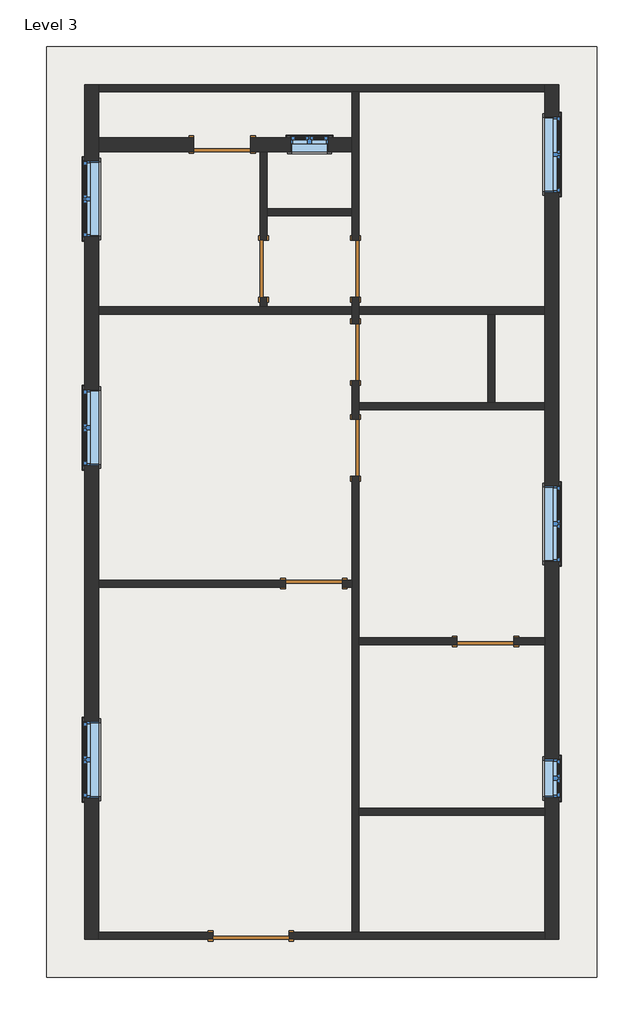
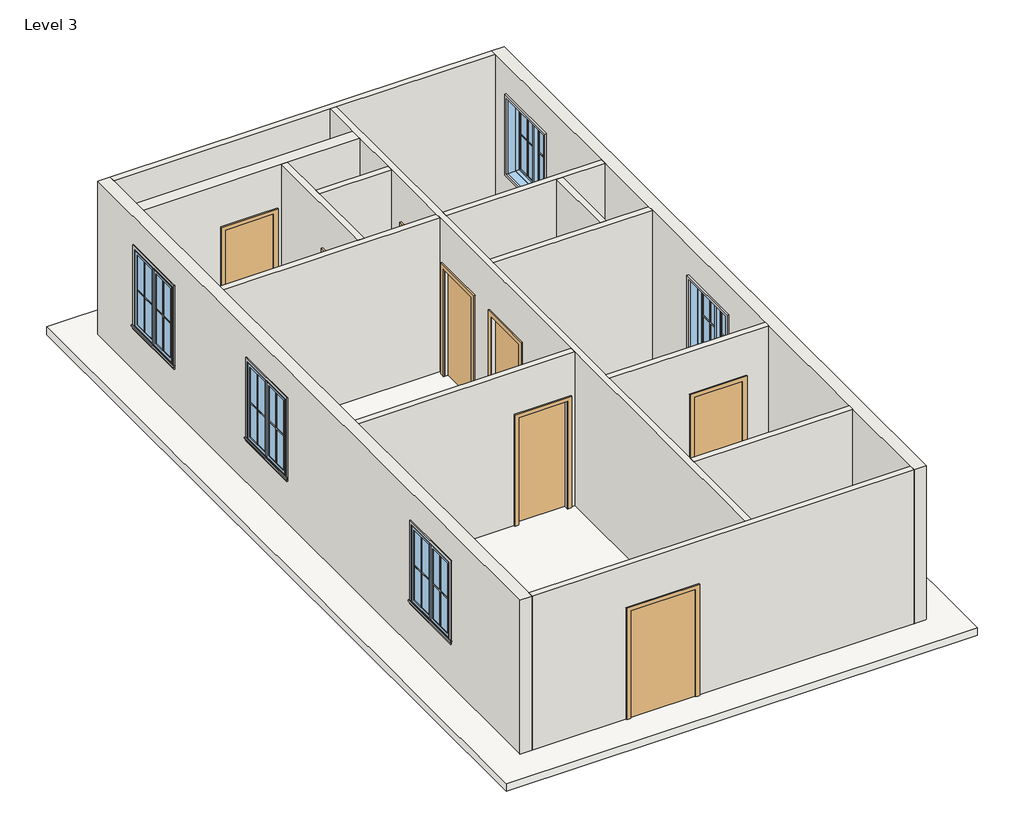
# One storey, incomplete: 28 proxies, 15 walls, 8 doors, 7 windows, 1 slab.
"""IFC4 building model written with IfcOpenShell, lengths in millimetres."""

from ifc_helpers import new_model, si_unit, frame, origin, place, context, project, spatial, polyline, outline, extrude, faceted_brep, transform, mapped, element, save
from components import muntin_pattern_2x2_muntin_pattern_2x2_6dad3731, muntin_pattern_2x2_muntin_pattern_2x2_a30a3345, muntin_pattern_2x2_muntin_pattern_2x2_53152e2c, muntin_pattern_2x2_muntin_pattern_2x2_e8f3e573, trim_window_exterior_flat_with_sill_92b9b949, trim_window_exterior_flat_with_sill_a665a915, trim_window_interior_flat_picture_frame_3bb882cf, trim_window_interior_flat_picture_frame_d485c387, door_a90ba1ad, door_e5f9f3c4, door_305aa2a5, door_6ea84ebe, window_c417fced, window_8377141f

model = new_model("IFC4")

# Units and contexts
model_context = context("Model", 3, world=origin())
ifc_project = project(units=[si_unit("LENGTHUNIT", "METRE", prefix="MILLI")], contexts=[model_context])

# Site, building, storey
site = spatial("IfcSite", under=ifc_project)
building = spatial("IfcBuilding", under=site)
storey = spatial("IfcBuildingStorey", under=building, Name="Level 3", Elevation=6096.0)

# Proxies
placement = place(None, origin())
muntin_pattern_2x2_muntin_pattern_2x2_shape = muntin_pattern_2x2_muntin_pattern_2x2_6dad3731(model_context)
element("IfcBuildingElementProxy", 1, Name="Muntin Pattern_2x2 : Muntin Pattern_2x2", ObjectType="Muntin Pattern_2x2 : Muntin Pattern_2x2", at=placement, inside=storey, context=model_context, shape_type="MappedRepresentation", body=[
    mapped(muntin_pattern_2x2_muntin_pattern_2x2_shape, transform((1279.525, 8669.3375, 7080.25), x_axis=(0.0, 1.0, 0.0), y_axis=(-1.0, 0.0, 0.0), z_axis=(0.0, 0.0, 1.0))),
])
element("IfcBuildingElementProxy", 2, Name="Muntin Pattern_2x2 : Muntin Pattern_2x2", ObjectType="Muntin Pattern_2x2 : Muntin Pattern_2x2", at=placement, inside=storey, context=model_context, shape_type="MappedRepresentation", body=[
    mapped(muntin_pattern_2x2_muntin_pattern_2x2_shape, transform((1279.525, 3341.6875, 7080.25), x_axis=(0.0, 1.0, 0.0), y_axis=(-1.0, 0.0, 0.0), z_axis=(0.0, 0.0, 1.0))),
])
element("IfcBuildingElementProxy", 3, Name="Muntin Pattern_2x2 : Muntin Pattern_2x2", ObjectType="Muntin Pattern_2x2 : Muntin Pattern_2x2", at=placement, inside=storey, context=model_context, shape_type="MappedRepresentation", body=[
    mapped(muntin_pattern_2x2_muntin_pattern_2x2_shape, transform((8880.475, 7732.7125, 7080.25), x_axis=(0.0, -1.0, 0.0), y_axis=(1.0, 0.0, 0.0), z_axis=(0.0, 0.0, 1.0))),
])
element("IfcBuildingElementProxy", 4, Name="Muntin Pattern_2x2 : Muntin Pattern_2x2", ObjectType="Muntin Pattern_2x2 : Muntin Pattern_2x2", at=placement, inside=storey, context=model_context, shape_type="MappedRepresentation", body=[
    mapped(muntin_pattern_2x2_muntin_pattern_2x2_shape, transform((8880.475, 13657.2625, 7080.25), x_axis=(0.0, -1.0, 0.0), y_axis=(1.0, 0.0, 0.0), z_axis=(0.0, 0.0, 1.0))),
])
element("IfcBuildingElementProxy", 5, Name="Muntin Pattern_2x2 : Muntin Pattern_2x2", ObjectType="Muntin Pattern_2x2 : Muntin Pattern_2x2", at=placement, inside=storey, context=model_context, shape_type="MappedRepresentation", body=[
    mapped(muntin_pattern_2x2_muntin_pattern_2x2_shape, transform((1279.525, 12339.6375, 7080.25), x_axis=(0.0, 1.0, 0.0), y_axis=(-1.0, 0.0, 0.0), z_axis=(0.0, 0.0, 1.0))),
])
muntin_pattern_2x2_muntin_pattern_2x2_2_shape = muntin_pattern_2x2_muntin_pattern_2x2_a30a3345(model_context)
element("IfcBuildingElementProxy", 6, Name="Muntin Pattern_2x2 : Muntin Pattern_2x2", ObjectType="Muntin Pattern_2x2 : Muntin Pattern_2x2", at=placement, inside=storey, context=model_context, shape_type="MappedRepresentation", body=[
    mapped(muntin_pattern_2x2_muntin_pattern_2x2_2_shape, transform((1279.525, 9275.7625, 7080.25), x_axis=(0.0, -1.0, 0.0), y_axis=(1.0, 0.0, 0.0), z_axis=(0.0, 0.0, 1.0))),
])
element("IfcBuildingElementProxy", 7, Name="Muntin Pattern_2x2 : Muntin Pattern_2x2", ObjectType="Muntin Pattern_2x2 : Muntin Pattern_2x2", at=placement, inside=storey, context=model_context, shape_type="MappedRepresentation", body=[
    mapped(muntin_pattern_2x2_muntin_pattern_2x2_2_shape, transform((1279.525, 3948.1125, 7080.25), x_axis=(0.0, -1.0, 0.0), y_axis=(1.0, 0.0, 0.0), z_axis=(0.0, 0.0, 1.0))),
])
element("IfcBuildingElementProxy", 8, Name="Muntin Pattern_2x2 : Muntin Pattern_2x2", ObjectType="Muntin Pattern_2x2 : Muntin Pattern_2x2", at=placement, inside=storey, context=model_context, shape_type="MappedRepresentation", body=[
    mapped(muntin_pattern_2x2_muntin_pattern_2x2_2_shape, transform((8880.475, 7126.2875, 7080.25), x_axis=(0.0, 1.0, 0.0), y_axis=(-1.0, 0.0, 0.0), z_axis=(0.0, 0.0, 1.0))),
])
element("IfcBuildingElementProxy", 9, Name="Muntin Pattern_2x2 : Muntin Pattern_2x2", ObjectType="Muntin Pattern_2x2 : Muntin Pattern_2x2", at=placement, inside=storey, context=model_context, shape_type="MappedRepresentation", body=[
    mapped(muntin_pattern_2x2_muntin_pattern_2x2_2_shape, transform((8880.475, 13050.8375, 7080.25), x_axis=(0.0, 1.0, 0.0), y_axis=(-1.0, 0.0, 0.0), z_axis=(0.0, 0.0, 1.0))),
])
element("IfcBuildingElementProxy", 10, Name="Muntin Pattern_2x2 : Muntin Pattern_2x2", ObjectType="Muntin Pattern_2x2 : Muntin Pattern_2x2", at=placement, inside=storey, context=model_context, shape_type="MappedRepresentation", body=[
    mapped(muntin_pattern_2x2_muntin_pattern_2x2_2_shape, transform((1279.525, 12946.0625, 7080.25), x_axis=(0.0, -1.0, 0.0), y_axis=(1.0, 0.0, 0.0), z_axis=(0.0, 0.0, 1.0))),
])
muntin_pattern_2x2_muntin_pattern_2x2_3_shape = muntin_pattern_2x2_muntin_pattern_2x2_53152e2c(model_context)
element("IfcBuildingElementProxy", 11, Name="Muntin Pattern_2x2 : Muntin Pattern_2x2", ObjectType="Muntin Pattern_2x2 : Muntin Pattern_2x2", at=placement, inside=storey, context=model_context, shape_type="MappedRepresentation", body=[
    mapped(muntin_pattern_2x2_muntin_pattern_2x2_3_shape, transform((4732.3375, 13617.575, 7080.25), x_axis=(1.0, 0.0, 0.0), y_axis=(0.0, 1.0, 0.0), z_axis=(0.0, 0.0, 1.0))),
])
element("IfcBuildingElementProxy", 12, Name="Muntin Pattern_2x2 : Muntin Pattern_2x2", ObjectType="Muntin Pattern_2x2 : Muntin Pattern_2x2", at=placement, inside=storey, context=model_context, shape_type="MappedRepresentation", body=[
    mapped(muntin_pattern_2x2_muntin_pattern_2x2_3_shape, transform((8880.475, 3497.2625, 7080.25), x_axis=(0.0, -1.0, 0.0), y_axis=(1.0, 0.0, 0.0), z_axis=(0.0, 0.0, 1.0))),
])
muntin_pattern_2x2_muntin_pattern_2x2_4_shape = muntin_pattern_2x2_muntin_pattern_2x2_e8f3e573(model_context)
element("IfcBuildingElementProxy", 13, Name="Muntin Pattern_2x2 : Muntin Pattern_2x2", ObjectType="Muntin Pattern_2x2 : Muntin Pattern_2x2", at=placement, inside=storey, context=model_context, shape_type="MappedRepresentation", body=[
    mapped(muntin_pattern_2x2_muntin_pattern_2x2_4_shape, transform((5033.9625, 13617.575, 7080.25), x_axis=(-1.0, 0.0, 0.0), y_axis=(0.0, -1.0, 0.0), z_axis=(0.0, 0.0, 1.0))),
])
element("IfcBuildingElementProxy", 14, Name="Muntin Pattern_2x2 : Muntin Pattern_2x2", ObjectType="Muntin Pattern_2x2 : Muntin Pattern_2x2", at=placement, inside=storey, context=model_context, shape_type="MappedRepresentation", body=[
    mapped(muntin_pattern_2x2_muntin_pattern_2x2_4_shape, transform((8880.475, 3195.6375, 7080.25), x_axis=(0.0, 1.0, 0.0), y_axis=(-1.0, 0.0, 0.0), z_axis=(0.0, 0.0, 1.0))),
])
trim_window_exterior_flat_with_sill_shape = trim_window_exterior_flat_with_sill_92b9b949(model_context)
element("IfcBuildingElementProxy", 15, Name="Trim-Window-Exterior-Flat : with Sill", ObjectType="Trim-Window-Exterior-Flat : with Sill", at=placement, inside=storey, context=model_context, shape_type="MappedRepresentation", body=[
    mapped(trim_window_exterior_flat_with_sill_shape, transform((1270.0, 8972.55, 8534.4), x_axis=(0.0, -1.0, 0.0), y_axis=(0.0, 0.0, 1.0), z_axis=(-1.0, 0.0, 0.0))),
])
element("IfcBuildingElementProxy", 16, Name="Trim-Window-Exterior-Flat : with Sill", ObjectType="Trim-Window-Exterior-Flat : with Sill", at=placement, inside=storey, context=model_context, shape_type="MappedRepresentation", body=[
    mapped(trim_window_exterior_flat_with_sill_shape, transform((1270.0, 3644.9, 8534.4), x_axis=(0.0, -1.0, 0.0), y_axis=(0.0, 0.0, 1.0), z_axis=(-1.0, 0.0, 0.0))),
])
element("IfcBuildingElementProxy", 17, Name="Trim-Window-Exterior-Flat : with Sill", ObjectType="Trim-Window-Exterior-Flat : with Sill", at=placement, inside=storey, context=model_context, shape_type="MappedRepresentation", body=[
    mapped(trim_window_exterior_flat_with_sill_shape, transform((8890.0, 7429.5, 8534.4), x_axis=(0.0, 1.0, 0.0), y_axis=(0.0, 0.0, 1.0), z_axis=(1.0, 0.0, 0.0))),
])
element("IfcBuildingElementProxy", 18, Name="Trim-Window-Exterior-Flat : with Sill", ObjectType="Trim-Window-Exterior-Flat : with Sill", at=placement, inside=storey, context=model_context, shape_type="MappedRepresentation", body=[
    mapped(trim_window_exterior_flat_with_sill_shape, transform((8890.0, 13354.05, 8534.4), x_axis=(0.0, 1.0, 0.0), y_axis=(0.0, 0.0, 1.0), z_axis=(1.0, 0.0, 0.0))),
])
element("IfcBuildingElementProxy", 19, Name="Trim-Window-Exterior-Flat : with Sill", ObjectType="Trim-Window-Exterior-Flat : with Sill", at=placement, inside=storey, context=model_context, shape_type="MappedRepresentation", body=[
    mapped(trim_window_exterior_flat_with_sill_shape, transform((1270.0, 12642.85, 8534.4), x_axis=(0.0, -1.0, 0.0), y_axis=(0.0, 0.0, 1.0), z_axis=(-1.0, 0.0, 0.0))),
])
trim_window_exterior_flat_with_sill_2_shape = trim_window_exterior_flat_with_sill_a665a915(model_context)
element("IfcBuildingElementProxy", 20, Name="Trim-Window-Exterior-Flat : with Sill", ObjectType="Trim-Window-Exterior-Flat : with Sill", at=placement, inside=storey, context=model_context, shape_type="MappedRepresentation", body=[
    mapped(trim_window_exterior_flat_with_sill_2_shape, transform((4883.15, 13627.1, 7924.8), x_axis=(-1.0, 0.0, 0.0), y_axis=(0.0, 0.0, 1.0), z_axis=(0.0, 1.0, 0.0))),
])
element("IfcBuildingElementProxy", 21, Name="Trim-Window-Exterior-Flat : with Sill", ObjectType="Trim-Window-Exterior-Flat : with Sill", at=placement, inside=storey, context=model_context, shape_type="MappedRepresentation", body=[
    mapped(trim_window_exterior_flat_with_sill_2_shape, transform((8890.0, 3346.45, 7924.8), x_axis=(0.0, 1.0, 0.0), y_axis=(0.0, 0.0, 1.0), z_axis=(1.0, 0.0, 0.0))),
])
trim_window_interior_flat_picture_frame_shape = trim_window_interior_flat_picture_frame_3bb882cf(model_context)
element("IfcBuildingElementProxy", 22, Name="Trim-Window-Interior-Flat : Picture Frame", ObjectType="Trim-Window-Interior-Flat : Picture Frame", at=placement, inside=storey, context=model_context, shape_type="MappedRepresentation", body=[
    mapped(trim_window_interior_flat_picture_frame_shape, transform((1498.6, 8972.55, 8534.4), x_axis=(0.0, 1.0, 0.0), y_axis=(0.0, 0.0, 1.0), z_axis=(1.0, 0.0, 0.0))),
])
element("IfcBuildingElementProxy", 23, Name="Trim-Window-Interior-Flat : Picture Frame", ObjectType="Trim-Window-Interior-Flat : Picture Frame", at=placement, inside=storey, context=model_context, shape_type="MappedRepresentation", body=[
    mapped(trim_window_interior_flat_picture_frame_shape, transform((1498.6, 3644.9, 8534.4), x_axis=(0.0, 1.0, 0.0), y_axis=(0.0, 0.0, 1.0), z_axis=(1.0, 0.0, 0.0))),
])
element("IfcBuildingElementProxy", 24, Name="Trim-Window-Interior-Flat : Picture Frame", ObjectType="Trim-Window-Interior-Flat : Picture Frame", at=placement, inside=storey, context=model_context, shape_type="MappedRepresentation", body=[
    mapped(trim_window_interior_flat_picture_frame_shape, transform((8661.4, 7429.5, 8534.4), x_axis=(0.0, -1.0, 0.0), y_axis=(0.0, 0.0, 1.0), z_axis=(-1.0, 0.0, 0.0))),
])
element("IfcBuildingElementProxy", 25, Name="Trim-Window-Interior-Flat : Picture Frame", ObjectType="Trim-Window-Interior-Flat : Picture Frame", at=placement, inside=storey, context=model_context, shape_type="MappedRepresentation", body=[
    mapped(trim_window_interior_flat_picture_frame_shape, transform((8661.4, 13354.05, 8534.4), x_axis=(0.0, -1.0, 0.0), y_axis=(0.0, 0.0, 1.0), z_axis=(-1.0, 0.0, 0.0))),
])
element("IfcBuildingElementProxy", 26, Name="Trim-Window-Interior-Flat : Picture Frame", ObjectType="Trim-Window-Interior-Flat : Picture Frame", at=placement, inside=storey, context=model_context, shape_type="MappedRepresentation", body=[
    mapped(trim_window_interior_flat_picture_frame_shape, transform((1498.6, 12642.85, 8534.4), x_axis=(0.0, 1.0, 0.0), y_axis=(0.0, 0.0, 1.0), z_axis=(1.0, 0.0, 0.0))),
])
trim_window_interior_flat_picture_frame_2_shape = trim_window_interior_flat_picture_frame_d485c387(model_context)
element("IfcBuildingElementProxy", 27, Name="Trim-Window-Interior-Flat : Picture Frame", ObjectType="Trim-Window-Interior-Flat : Picture Frame", at=placement, inside=storey, context=model_context, shape_type="MappedRepresentation", body=[
    mapped(trim_window_interior_flat_picture_frame_2_shape, transform((4883.15, 13398.5, 7924.8), x_axis=(1.0, 0.0, 0.0), y_axis=(0.0, 0.0, 1.0), z_axis=(0.0, -1.0, 0.0))),
])
element("IfcBuildingElementProxy", 28, Name="Trim-Window-Interior-Flat : Picture Frame", ObjectType="Trim-Window-Interior-Flat : Picture Frame", at=placement, inside=storey, context=model_context, shape_type="MappedRepresentation", body=[
    mapped(trim_window_interior_flat_picture_frame_2_shape, transform((8661.4, 3346.45, 7924.8), x_axis=(0.0, -1.0, 0.0), y_axis=(0.0, 0.0, 1.0), z_axis=(-1.0, 0.0, 0.0))),
])

# Doors
door_shape = door_a90ba1ad(model_context)
element("IfcDoor", 29, ObjectType="Single-Flush : 36\" x 84\"", at=placement, inside=storey, context=model_context, shape_type="MappedRepresentation", body=[
    mapped(door_shape, transform((3479.8, 13512.8, 6096.0), x_axis=(1.0, 0.0, 0.0), y_axis=(0.0, 1.0, 0.0), z_axis=(0.0, 0.0, 1.0))),
])
door_2_shape = door_e5f9f3c4(model_context)
element("IfcDoor", 30, ObjectType="Single-Flush : 36\" x 84\"", at=placement, inside=storey, context=model_context, shape_type="MappedRepresentation", body=[
    mapped(door_2_shape, transform((5619.75, 11518.9, 6096.0), x_axis=(0.0, -1.0, 0.0), y_axis=(1.0, 0.0, 0.0), z_axis=(0.0, 0.0, 1.0))),
])
element("IfcDoor", 31, ObjectType="Single-Flush : 36\" x 84\"", at=placement, inside=storey, context=model_context, shape_type="MappedRepresentation", body=[
    mapped(door_2_shape, transform((4953.0, 6470.65, 6096.0), x_axis=(1.0, 0.0, 0.0), y_axis=(0.0, 1.0, 0.0), z_axis=(0.0, 0.0, 1.0))),
])
element("IfcDoor", 32, ObjectType="Single-Flush : 36\" x 84\"", at=placement, inside=storey, context=model_context, shape_type="MappedRepresentation", body=[
    mapped(door_2_shape, transform((7708.9, 5543.55, 6096.0), x_axis=(-1.0, 0.0, 0.0), y_axis=(0.0, -1.0, 0.0), z_axis=(0.0, 0.0, 1.0))),
])
door_3_shape = door_305aa2a5(model_context)
element("IfcDoor", 33, ObjectType="Single-Flush : 36\" x 84\"", at=placement, inside=storey, context=model_context, shape_type="MappedRepresentation", body=[
    mapped(door_3_shape, transform((4146.55, 11518.9, 6096.0), x_axis=(0.0, -1.0, 0.0), y_axis=(1.0, 0.0, 0.0), z_axis=(0.0, 0.0, 1.0))),
])
element("IfcDoor", 34, ObjectType="Single-Flush : 36\" x 84\"", at=placement, inside=storey, context=model_context, shape_type="MappedRepresentation", body=[
    mapped(door_3_shape, transform((5619.75, 10185.4, 6096.0), x_axis=(0.0, 1.0, 0.0), y_axis=(-1.0, 0.0, 0.0), z_axis=(0.0, 0.0, 1.0))),
])
element("IfcDoor", 35, ObjectType="Single-Flush : 36\" x 84\"", at=placement, inside=storey, context=model_context, shape_type="MappedRepresentation", body=[
    mapped(door_3_shape, transform((5619.75, 8648.7, 6096.0), x_axis=(0.0, 1.0, 0.0), y_axis=(-1.0, 0.0, 0.0), z_axis=(0.0, 0.0, 1.0))),
])
door_4_shape = door_6ea84ebe(model_context)
element("IfcDoor", 36, ObjectType="Single-Flush : 48\" x 84\"", at=placement, inside=storey, context=model_context, shape_type="MappedRepresentation", body=[
    mapped(door_4_shape, transform((3943.35, 819.15, 6096.0), x_axis=(-1.0, 0.0, 0.0), y_axis=(0.0, -1.0, 0.0), z_axis=(0.0, 0.0, 1.0))),
])

# Slab
element("IfcSlab", 37, ObjectType="Generic - 12\"", at=placement, inside=storey, context=model_context, shape_type="SweptSolid", body=[
    extrude(outline(polyline([(9499.6, 15087.6), (9499.6, 152.4), (660.4, 152.4), (660.4, 15087.6), (9499.6, 15087.6)])), frame((0.0, 0.0, 5943.6), z_axis=(0.0, 0.0, 1.0), x_axis=(1.0, 0.0, 0.0)), (0.0, 0.0, 1.0), 152.4),
])

# Walls
element("IfcWall", 38, ObjectType="Generic - 5\"", at=placement, inside=storey, context=model_context, shape_type="Brep", body=[
    faceted_brep([(1498.6, 14363.7, 6096.0), (5562.6, 14363.7, 6096.0), (5676.9, 14363.7, 6096.0), (8661.4, 14363.7, 6096.0), (8661.4, 14363.7, 9144.0), (5676.9, 14363.7, 9144.0), (5562.6, 14363.7, 9144.0), (1498.6, 14363.7, 9144.0), (1498.6, 14478.0, 6096.0), (1498.6, 14478.0, 9144.0), (8661.4, 14478.0, 9144.0), (8661.4, 14478.0, 6096.0)], [[[0, 1, 2, 3, 4, 5, 6, 7]], [[8, 9, 10, 11]], [[3, 2, 1, 0, 8, 11]], [[7, 6, 5, 4, 10, 9]], [[4, 3, 11, 10]], [[0, 7, 9, 8]]]),
])
element("IfcWall", 39, ObjectType="Generic - 5\"", at=placement, inside=storey, context=model_context, shape_type="Brep", body=[
    faceted_brep([(1498.6, 762.0, 6096.0), (3333.75, 762.0, 6096.0), (3333.75, 762.0, 8229.6), (4552.95, 762.0, 8229.6), (4552.95, 762.0, 6096.0), (8661.4, 762.0, 6096.0), (8661.4, 762.0, 9144.0), (1498.6, 762.0, 9144.0), (3333.75, 876.3, 8229.6), (3333.75, 876.3, 6096.0), (1498.6, 876.3, 6096.0), (1498.6, 876.3, 9144.0), (5562.6, 876.3, 9144.0), (5676.9, 876.3, 9144.0), (8661.4, 876.3, 9144.0), (8661.4, 876.3, 6096.0), (5676.9, 876.3, 6096.0), (5562.6, 876.3, 6096.0), (4552.95, 876.3, 6096.0), (4552.95, 876.3, 8229.6)], [[[0, 1, 2, 3, 4, 5, 6, 7]], [[8, 9, 10, 11, 12, 13, 14, 15, 16, 17, 18, 19]], [[10, 9, 1, 0]], [[18, 17, 16, 15, 5, 4]], [[7, 6, 14, 13, 12, 11]], [[6, 5, 15, 14]], [[0, 7, 11, 10]], [[2, 1, 9, 8]], [[3, 2, 8, 19]], [[4, 3, 19, 18]]]),
])
element("IfcWall", 40, ObjectType="Generic - 5\"", at=placement, inside=storey, context=model_context, shape_type="Brep", body=[
    faceted_brep([(5562.6, 9728.2, 6096.0), (5562.6, 9105.9, 6096.0), (5562.6, 9105.9, 8229.6), (5562.6, 8191.5, 8229.6), (5562.6, 8191.5, 6096.0), (5562.6, 6527.8, 6096.0), (5562.6, 6413.5, 6096.0), (5562.6, 876.3, 6096.0), (5562.6, 876.3, 9144.0), (5562.6, 6413.5, 9144.0), (5562.6, 6527.8, 9144.0), (5562.6, 10795.0, 9144.0), (5562.6, 10909.3, 9144.0), (5562.6, 12369.8, 9144.0), (5562.6, 12484.1, 9144.0), (5562.6, 13398.5, 9144.0), (5562.6, 13627.1, 9144.0), (5562.6, 14363.7, 9144.0), (5562.6, 14363.7, 6096.0), (5562.6, 13627.1, 6096.0), (5562.6, 13398.5, 6096.0), (5562.6, 12484.1, 6096.0), (5562.6, 12369.8, 6096.0), (5562.6, 11976.1, 6096.0), (5562.6, 11976.1, 8229.6), (5562.6, 11061.7, 8229.6), (5562.6, 11061.7, 6096.0), (5562.6, 10909.3, 6096.0), (5562.6, 10795.0, 6096.0), (5562.6, 10642.6, 6096.0), (5562.6, 10642.6, 8229.6), (5562.6, 9728.2, 8229.6), (5676.9, 9105.9, 8229.6), (5676.9, 9105.9, 6096.0), (5676.9, 9258.3, 6096.0), (5676.9, 9372.6, 6096.0), (5676.9, 9728.2, 6096.0), (5676.9, 9728.2, 8229.6), (5676.9, 10642.6, 8229.6), (5676.9, 10642.6, 6096.0), (5676.9, 10795.0, 6096.0), (5676.9, 10909.3, 6096.0), (5676.9, 11061.7, 6096.0), (5676.9, 11061.7, 8229.6), (5676.9, 11976.1, 8229.6), (5676.9, 11976.1, 6096.0), (5676.9, 14363.7, 6096.0), (5676.9, 14363.7, 9144.0), (5676.9, 10909.3, 9144.0), (5676.9, 10795.0, 9144.0), (5676.9, 9372.6, 9144.0), (5676.9, 9258.3, 9144.0), (5676.9, 5600.7, 9144.0), (5676.9, 5486.4, 9144.0), (5676.9, 2870.2, 9144.0), (5676.9, 2755.9, 9144.0), (5676.9, 876.3, 9144.0), (5676.9, 876.3, 6096.0), (5676.9, 2755.9, 6096.0), (5676.9, 2870.2, 6096.0), (5676.9, 5486.4, 6096.0), (5676.9, 5600.7, 6096.0), (5676.9, 8191.5, 6096.0), (5676.9, 8191.5, 8229.6)], [[[0, 1, 2, 3, 4, 5, 6, 7, 8, 9, 10, 11, 12, 13, 14, 15, 16, 17, 18, 19, 20, 21, 22, 23, 24, 25, 26, 27, 28, 29, 30, 31]], [[32, 33, 34, 35, 36, 37, 38, 39, 40, 41, 42, 43, 44, 45, 46, 47, 48, 49, 50, 51, 52, 53, 54, 55, 56, 57, 58, 59, 60, 61, 62, 63]], [[23, 22, 21, 20, 19, 18, 46, 45]], [[42, 41, 40, 39, 29, 28, 27, 26]], [[36, 35, 34, 33, 1, 0]], [[62, 61, 60, 59, 58, 57, 7, 6, 5, 4]], [[17, 16, 15, 14, 13, 12, 11, 10, 9, 8, 56, 55, 54, 53, 52, 51, 50, 49, 48, 47]], [[18, 17, 47, 46]], [[8, 7, 57, 56]], [[43, 42, 26, 25]], [[44, 43, 25, 24]], [[45, 44, 24, 23]], [[30, 29, 39, 38]], [[31, 30, 38, 37]], [[0, 31, 37, 36]], [[2, 1, 33, 32]], [[3, 2, 32, 63]], [[4, 3, 63, 62]]]),
])
element("IfcWall", 41, ObjectType="Generic - 5\"", at=placement, inside=storey, context=model_context, shape_type="SweptSolid", body=[
    extrude(outline(polyline([(6096.0, 5676.9), (6096.0, 7251.7), (8229.6, 7251.7), (8229.6, 8166.1), (6096.0, 8166.1), (6096.0, 8661.4), (9144.0, 8661.4), (9144.0, 5676.9), (6096.0, 5676.9)])), frame((0.0, 5486.4, 0.0), z_axis=(0.0, 1.0, 0.0), x_axis=(0.0, 0.0, 1.0)), (0.0, 0.0, 1.0), 114.3),
])
element("IfcWall", 42, ObjectType="Generic - 5\"", at=placement, inside=storey, context=model_context, shape_type="SweptSolid", body=[
    extrude(outline(polyline([(8229.6, 5410.2), (6096.0, 5410.2), (6096.0, 5562.6), (9144.0, 5562.6), (9144.0, 1498.6), (6096.0, 1498.6), (6096.0, 4495.8), (8229.6, 4495.8), (8229.6, 5410.2)])), frame((0.0, 6413.5, 0.0), z_axis=(0.0, 1.0, 0.0), x_axis=(0.0, 0.0, 1.0)), (0.0, 0.0, 1.0), 114.3),
])
element("IfcWall", 43, ObjectType="Generic - 5\"", at=placement, inside=storey, context=model_context, shape_type="Brep", body=[
    faceted_brep([(1498.6, 10795.0, 6096.0), (5562.6, 10795.0, 6096.0), (5562.6, 10795.0, 9144.0), (1498.6, 10795.0, 9144.0), (1498.6, 10909.3, 6096.0), (1498.6, 10909.3, 9144.0), (4089.4, 10909.3, 9144.0), (4203.7, 10909.3, 9144.0), (5562.6, 10909.3, 9144.0), (5562.6, 10909.3, 6096.0), (4203.7, 10909.3, 6096.0), (4089.4, 10909.3, 6096.0)], [[[0, 1, 2, 3]], [[4, 5, 6, 7, 8, 9, 10, 11]], [[1, 0, 4, 11, 10, 9]], [[3, 2, 8, 7, 6, 5]], [[0, 3, 5, 4]], [[2, 1, 9, 8]]]),
])
element("IfcWall", 44, ObjectType="Generic - 5\"", at=placement, inside=storey, context=model_context, shape_type="Brep", body=[
    faceted_brep([(5676.9, 10795.0, 6096.0), (7747.0010433, 10795.0, 6096.0), (7861.3010433, 10795.0, 6096.0), (8661.4, 10795.0, 6096.0), (8661.4, 10795.0, 9144.0), (7861.3010433, 10795.0, 9144.0), (7747.0010433, 10795.0, 9144.0), (5676.9, 10795.0, 9144.0), (5676.9, 10909.3, 6096.0), (5676.9, 10909.3, 9144.0), (8661.4, 10909.3, 9144.0), (8661.4, 10909.3, 6096.0)], [[[0, 1, 2, 3, 4, 5, 6, 7]], [[8, 9, 10, 11]], [[3, 2, 1, 0, 8, 11]], [[7, 6, 5, 4, 10, 9]], [[4, 3, 11, 10]], [[0, 7, 9, 8]]]),
])
element("IfcWall", 45, ObjectType="Generic - 5\"", at=placement, inside=storey, context=model_context, shape_type="SweptSolid", body=[
    extrude(outline(polyline([(7747.0010433, 9372.6), (7747.0010433, 10795.0), (7861.3010433, 10795.0), (7861.3010433, 9372.6), (7747.0010433, 9372.6)])), frame((0.0, 0.0, 6096.0), z_axis=(0.0, 0.0, 1.0), x_axis=(1.0, 0.0, 0.0)), (0.0, 0.0, 1.0), 3048.0),
])
element("IfcWall", 46, ObjectType="Generic - 5\"", at=placement, inside=storey, context=model_context, shape_type="Brep", body=[
    faceted_brep([(5676.9, 9258.3, 6096.0), (8661.4, 9258.3, 6096.0), (8661.4, 9258.3, 9144.0), (5676.9, 9258.3, 9144.0), (5676.9, 9372.6, 6096.0), (5676.9, 9372.6, 9144.0), (7747.0010433, 9372.6, 9144.0), (7861.3010433, 9372.6, 9144.0), (8661.4, 9372.6, 9144.0), (8661.4, 9372.6, 6096.0), (7861.3010433, 9372.6, 6096.0), (7747.0010433, 9372.6, 6096.0)], [[[0, 1, 2, 3]], [[4, 5, 6, 7, 8, 9, 10, 11]], [[1, 0, 4, 11, 10, 9]], [[3, 2, 8, 7, 6, 5]], [[2, 1, 9, 8]], [[0, 3, 5, 4]]]),
])
element("IfcWall", 47, ObjectType="Generic - 5\"", at=placement, inside=storey, context=model_context, shape_type="SweptSolid", body=[
    extrude(outline(polyline([(8661.4, 2755.9), (5676.9, 2755.9), (5676.9, 2870.2), (8661.4, 2870.2), (8661.4, 2755.9)])), frame((0.0, 0.0, 6096.0), z_axis=(0.0, 0.0, 1.0), x_axis=(1.0, 0.0, 0.0)), (0.0, 0.0, 1.0), 3048.0),
])
element("IfcWall", 48, ObjectType="Generic - 5\"", at=placement, inside=storey, context=model_context, shape_type="Brep", body=[
    faceted_brep([(4203.7, 10909.3, 6096.0), (4203.7, 11061.7, 6096.0), (4203.7, 11061.7, 8229.6), (4203.7, 11976.1, 8229.6), (4203.7, 11976.1, 6096.0), (4203.7, 12369.8, 6096.0), (4203.7, 12484.1, 6096.0), (4203.7, 13398.5, 6096.0), (4203.7, 13398.5, 9144.0), (4203.7, 12484.1, 9144.0), (4203.7, 12369.8, 9144.0), (4203.7, 10909.3, 9144.0), (4089.4, 11061.7, 8229.6), (4089.4, 11061.7, 6096.0), (4089.4, 10909.3, 6096.0), (4089.4, 10909.3, 9144.0), (4089.4, 13398.5, 9144.0), (4089.4, 13398.5, 6096.0), (4089.4, 11976.1, 6096.0), (4089.4, 11976.1, 8229.6)], [[[0, 1, 2, 3, 4, 5, 6, 7, 8, 9, 10, 11]], [[12, 13, 14, 15, 16, 17, 18, 19]], [[18, 17, 7, 6, 5, 4]], [[14, 13, 1, 0]], [[11, 10, 9, 8, 16, 15]], [[0, 11, 15, 14]], [[8, 7, 17, 16]], [[2, 1, 13, 12]], [[3, 2, 12, 19]], [[4, 3, 19, 18]]]),
])
element("IfcWall", 49, ObjectType="Generic - 5\"", at=placement, inside=storey, context=model_context, shape_type="SweptSolid", body=[
    extrude(outline(polyline([(5562.6, 12369.8), (4203.7, 12369.8), (4203.7, 12484.1), (5562.6, 12484.1), (5562.6, 12369.8)])), frame((0.0, 0.0, 6096.0), z_axis=(0.0, 0.0, 1.0), x_axis=(1.0, 0.0, 0.0)), (0.0, 0.0, 1.0), 3048.0),
])
element("IfcWall", 50, ObjectType="Generic - 8\"", at=placement, inside=storey, context=model_context, shape_type="Brep", body=[
    faceted_brep([(8661.4, 14478.0, 6096.0), (8661.4, 14363.7, 6096.0), (8661.4, 10909.3, 6096.0), (8661.4, 10795.0, 6096.0), (8661.4, 9372.6, 6096.0), (8661.4, 9258.3, 6096.0), (8661.4, 5600.7, 6096.0), (8661.4, 5486.4, 6096.0), (8661.4, 2870.2, 6096.0), (8661.4, 2755.9, 6096.0), (8661.4, 876.3, 6096.0), (8661.4, 762.0, 6096.0), (8661.4, 762.0, 9144.0), (8661.4, 876.3, 9144.0), (8661.4, 2755.9, 9144.0), (8661.4, 2870.2, 9144.0), (8661.4, 5486.4, 9144.0), (8661.4, 5600.7, 9144.0), (8661.4, 9258.3, 9144.0), (8661.4, 9372.6, 9144.0), (8661.4, 10795.0, 9144.0), (8661.4, 10909.3, 9144.0), (8661.4, 14363.7, 9144.0), (8661.4, 14478.0, 9144.0), (8661.4, 6819.9, 8534.4), (8661.4, 6819.9, 7010.4), (8661.4, 8039.1, 7010.4), (8661.4, 8039.1, 8534.4), (8661.4, 12744.45, 8534.4), (8661.4, 12744.45, 7010.4), (8661.4, 13963.65, 7010.4), (8661.4, 13963.65, 8534.4), (8661.4, 3041.65, 7924.8), (8661.4, 3041.65, 7010.4), (8661.4, 3651.25, 7010.4), (8661.4, 3651.25, 7924.8), (8890.0, 14478.0, 6096.0), (8890.0, 14478.0, 9144.0), (8890.0, 762.0, 9144.0), (8890.0, 762.0, 6096.0), (8890.0, 6819.9, 8534.4), (8890.0, 8039.1, 8534.4), (8890.0, 8039.1, 7010.4), (8890.0, 6819.9, 7010.4), (8890.0, 12744.45, 8534.4), (8890.0, 13963.65, 8534.4), (8890.0, 13963.65, 7010.4), (8890.0, 12744.45, 7010.4), (8890.0, 3041.65, 7924.8), (8890.0, 3651.25, 7924.8), (8890.0, 3651.25, 7010.4), (8890.0, 3041.65, 7010.4)], [[[0, 1, 2, 3, 4, 5, 6, 7, 8, 9, 10, 11, 12, 13, 14, 15, 16, 17, 18, 19, 20, 21, 22, 23], [24, 25, 26, 27], [28, 29, 30, 31], [32, 33, 34, 35]], [[36, 37, 38, 39], [40, 41, 42, 43], [44, 45, 46, 47], [48, 49, 50, 51]], [[11, 10, 9, 8, 7, 6, 5, 4, 3, 2, 1, 0, 36, 39]], [[23, 22, 21, 20, 19, 18, 17, 16, 15, 14, 13, 12, 38, 37]], [[0, 23, 37, 36]], [[12, 11, 39, 38]], [[25, 24, 40, 43]], [[26, 25, 43, 42]], [[27, 26, 42, 41]], [[24, 27, 41, 40]], [[29, 28, 44, 47]], [[30, 29, 47, 46]], [[31, 30, 46, 45]], [[28, 31, 45, 44]], [[33, 32, 48, 51]], [[34, 33, 51, 50]], [[35, 34, 50, 49]], [[32, 35, 49, 48]]]),
])
element("IfcWall", 51, ObjectType="Generic - 8\"", at=placement, inside=storey, context=model_context, shape_type="Brep", body=[
    faceted_brep([(1270.0, 14478.0, 6096.0), (1270.0, 762.0, 6096.0), (1270.0, 762.0, 9144.0), (1270.0, 14478.0, 9144.0), (1270.0, 9582.15, 8534.4), (1270.0, 8362.95, 8534.4), (1270.0, 8362.95, 7010.4), (1270.0, 9582.15, 7010.4), (1270.0, 4254.5, 8534.4), (1270.0, 3035.3, 8534.4), (1270.0, 3035.3, 7010.4), (1270.0, 4254.5, 7010.4), (1270.0, 13252.45, 8534.4), (1270.0, 12033.25, 8534.4), (1270.0, 12033.25, 7010.4), (1270.0, 13252.45, 7010.4), (1498.6, 14478.0, 6096.0), (1498.6, 14478.0, 9144.0), (1498.6, 14363.7, 9144.0), (1498.6, 13627.1, 9144.0), (1498.6, 13398.5, 9144.0), (1498.6, 10909.3, 9144.0), (1498.6, 10795.0, 9144.0), (1498.6, 6527.8, 9144.0), (1498.6, 6413.5, 9144.0), (1498.6, 876.3, 9144.0), (1498.6, 762.0, 9144.0), (1498.6, 762.0, 6096.0), (1498.6, 876.3, 6096.0), (1498.6, 6413.5, 6096.0), (1498.6, 6527.8, 6096.0), (1498.6, 10795.0, 6096.0), (1498.6, 10909.3, 6096.0), (1498.6, 13398.5, 6096.0), (1498.6, 13627.1, 6096.0), (1498.6, 14363.7, 6096.0), (1498.6, 9582.15, 8534.4), (1498.6, 9582.15, 7010.4), (1498.6, 8362.95, 7010.4), (1498.6, 8362.95, 8534.4), (1498.6, 4254.5, 8534.4), (1498.6, 4254.5, 7010.4), (1498.6, 3035.3, 7010.4), (1498.6, 3035.3, 8534.4), (1498.6, 13252.45, 8534.4), (1498.6, 13252.45, 7010.4), (1498.6, 12033.25, 7010.4), (1498.6, 12033.25, 8534.4)], [[[0, 1, 2, 3], [4, 5, 6, 7], [8, 9, 10, 11], [12, 13, 14, 15]], [[16, 17, 18, 19, 20, 21, 22, 23, 24, 25, 26, 27, 28, 29, 30, 31, 32, 33, 34, 35], [36, 37, 38, 39], [40, 41, 42, 43], [44, 45, 46, 47]], [[1, 0, 16, 35, 34, 33, 32, 31, 30, 29, 28, 27]], [[3, 2, 26, 25, 24, 23, 22, 21, 20, 19, 18, 17]], [[0, 3, 17, 16]], [[2, 1, 27, 26]], [[37, 36, 4, 7]], [[38, 37, 7, 6]], [[39, 38, 6, 5]], [[36, 39, 5, 4]], [[41, 40, 8, 11]], [[42, 41, 11, 10]], [[43, 42, 10, 9]], [[40, 43, 9, 8]], [[45, 44, 12, 15]], [[46, 45, 15, 14]], [[47, 46, 14, 13]], [[44, 47, 13, 12]]]),
])
element("IfcWall", 52, ObjectType="Generic - 8\"", at=placement, inside=storey, context=model_context, shape_type="Brep", body=[
    faceted_brep([(3937.0, 13398.5, 8229.6), (3937.0, 13398.5, 6096.0), (4089.4, 13398.5, 6096.0), (4203.7, 13398.5, 6096.0), (5562.6, 13398.5, 6096.0), (5562.6, 13398.5, 9144.0), (4203.7, 13398.5, 9144.0), (4089.4, 13398.5, 9144.0), (1498.6, 13398.5, 9144.0), (1498.6, 13398.5, 6096.0), (3022.6, 13398.5, 6096.0), (3022.6, 13398.5, 8229.6), (5187.95, 13398.5, 7924.8), (5187.95, 13398.5, 7010.4), (4578.35, 13398.5, 7010.4), (4578.35, 13398.5, 7924.8), (5562.6, 13627.1, 6096.0), (3937.0, 13627.1, 6096.0), (3937.0, 13627.1, 8229.6), (3022.6, 13627.1, 8229.6), (3022.6, 13627.1, 6096.0), (1498.6, 13627.1, 6096.0), (1498.6, 13627.1, 9144.0), (5562.6, 13627.1, 9144.0), (5187.95, 13627.1, 7924.8), (4578.35, 13627.1, 7924.8), (4578.35, 13627.1, 7010.4), (5187.95, 13627.1, 7010.4)], [[[0, 1, 2, 3, 4, 5, 6, 7, 8, 9, 10, 11], [12, 13, 14, 15]], [[16, 17, 18, 19, 20, 21, 22, 23], [24, 25, 26, 27]], [[10, 9, 21, 20]], [[4, 3, 2, 1, 17, 16]], [[8, 7, 6, 5, 23, 22]], [[9, 8, 22, 21]], [[5, 4, 16, 23]], [[18, 17, 1, 0]], [[19, 18, 0, 11]], [[20, 19, 11, 10]], [[13, 12, 24, 27]], [[14, 13, 27, 26]], [[15, 14, 26, 25]], [[12, 15, 25, 24]]]),
])

# Windows
window_shape = window_c417fced(model_context)
element("IfcWindow", 53, ObjectType="Window-Casement-Double : 24\" x 36\"", at=placement, inside=storey, context=model_context, shape_type="MappedRepresentation", body=[
    mapped(window_shape, transform((4883.15, 13512.8, 6096.0), x_axis=(1.0, 0.0, 0.0), y_axis=(0.0, 1.0, 0.0), z_axis=(0.0, 0.0, 1.0))),
])
element("IfcWindow", 54, ObjectType="Window-Casement-Double : 24\" x 36\"", at=placement, inside=storey, context=model_context, shape_type="MappedRepresentation", body=[
    mapped(window_shape, transform((8775.7, 3346.45, 6096.0), x_axis=(0.0, -1.0, 0.0), y_axis=(1.0, 0.0, 0.0), z_axis=(0.0, 0.0, 1.0))),
])
window_2_shape = window_8377141f(model_context)
element("IfcWindow", 55, ObjectType="Window-Casement-Double : 48\" x 60\"", at=placement, inside=storey, context=model_context, shape_type="MappedRepresentation", body=[
    mapped(window_2_shape, transform((1384.3, 8972.55, 6096.0), x_axis=(0.0, 1.0, 0.0), y_axis=(-1.0, 0.0, 0.0), z_axis=(0.0, 0.0, 1.0))),
])
element("IfcWindow", 56, ObjectType="Window-Casement-Double : 48\" x 60\"", at=placement, inside=storey, context=model_context, shape_type="MappedRepresentation", body=[
    mapped(window_2_shape, transform((1384.3, 3644.9, 6096.0), x_axis=(0.0, 1.0, 0.0), y_axis=(-1.0, 0.0, 0.0), z_axis=(0.0, 0.0, 1.0))),
])
element("IfcWindow", 57, ObjectType="Window-Casement-Double : 48\" x 60\"", at=placement, inside=storey, context=model_context, shape_type="MappedRepresentation", body=[
    mapped(window_2_shape, transform((8775.7, 7429.5, 6096.0), x_axis=(0.0, -1.0, 0.0), y_axis=(1.0, 0.0, 0.0), z_axis=(0.0, 0.0, 1.0))),
])
element("IfcWindow", 58, ObjectType="Window-Casement-Double : 48\" x 60\"", at=placement, inside=storey, context=model_context, shape_type="MappedRepresentation", body=[
    mapped(window_2_shape, transform((8775.7, 13354.05, 6096.0), x_axis=(0.0, -1.0, 0.0), y_axis=(1.0, 0.0, 0.0), z_axis=(0.0, 0.0, 1.0))),
])
element("IfcWindow", 59, ObjectType="Window-Casement-Double : 48\" x 60\"", at=placement, inside=storey, context=model_context, shape_type="MappedRepresentation", body=[
    mapped(window_2_shape, transform((1384.3, 12642.85, 6096.0), x_axis=(0.0, 1.0, 0.0), y_axis=(-1.0, 0.0, 0.0), z_axis=(0.0, 0.0, 1.0))),
])

save(model, "model.ifc")

# Revit data of these elements
# Type "Muntin Pattern_2x2 : Muntin Pattern_2x2"
#   Width [instance default] = 4' - 0"
#   Thickness = 0' - 0 1/2"
#   Height [instance default] = 4' - 0"
#   Distance = 0' - 0 3/4"
#   Interior Material [instance default] = none
#   Exterior Material [instance default] = none
#   Default Elevation = 0
# Type "Trim-Window-Exterior-Flat : with Sill"
#   Trim Width = 0' - 2 1/4"
#   Trim Thickness_Picture Frame = 0' - 1 1/4"
#   Trim Thickness_with Sill = 0' - 0 3/4"
#   Sill Thickness = 0' - 1 1/4"
#   Opening Width [instance default] = 2' - 0"
#   Opening Height [instance default] = 3' - 0"
#   Default Elevation = 4' - 0"
#   Sill = yes
#   Picture Frame = no
#   Trim Material [instance default] = none
# Type "Trim-Window-Interior-Flat : Picture Frame"
#   Trim Thickness_Picture Frame = 0' - 1 1/4"
#   Trim Width = 0' - 2 1/4"
#   Trim Thickness_with Sill = 0' - 0 3/4"
#   Sill Thickness = 0' - 1 1/4"
#   Opening Width [instance default] = 2' - 0"
#   Opening Height [instance default] = 3' - 0"
#   Default Elevation = 4' - 0"
#   Sill = no
#   Picture Frame = yes
#   Trim Material [instance default] = none
# Type "Single-Flush : 36\" x 84\""
#   Type Mark = "1"
#   Construction Type Id = "MDOOR"
#   Assembly Code = "C1020"
#   Analytic Construction = "Metal"
#   Thickness = 0' - 2"
#   Heat Transfer Coefficient (U) = 0.651978 BTU/(h·ft²·°F)
#   Height = 7' - 0"
#   Trim Projection Ext = 0' - 1"
#   Trim Projection Int = 0' - 1"
#   Trim Width = 0' - 3"
#   Width = 3' - 0"
#   Define Thermal Properties by = 1
#   Define Thermal Properties by = 1
#   Door Material = Door - Panel
#   Frame Material = Door - Frame
#   Visual Light Transmittance = 0
#   Solar Heat Gain Coefficient = 0
#   Function = (empty or 0)
#   Wall Closure = (empty or 0)
# Type "Single-Flush : 48\" x 84\""
#   Type Mark = "5"
#   Construction Type Id = "MDOOR"
#   Assembly Code = "C1020"
#   Analytic Construction = "Metal"
#   Thickness = 0' - 2"
#   Heat Transfer Coefficient (U) = 0.651978 BTU/(h·ft²·°F)
#   Height = 7' - 0"
#   Trim Projection Ext = 0' - 1"
#   Trim Projection Int = 0' - 1"
#   Trim Width = 0' - 3"
#   Width = 4' - 0"
#   Define Thermal Properties by = 1
#   Define Thermal Properties by = 1
#   Door Material = Door - Panel
#   Frame Material = Door - Frame
#   Visual Light Transmittance = 0
#   Solar Heat Gain Coefficient = 0
#   Function = (empty or 0)
#   Wall Closure = (empty or 0)
# Type "Generic - 12\""
#   Assembly Code = "B1010"
#   Function = 0
#   Layers, outside or top first: 0' - 6" no material (function 1)
# Type "Generic - 5\""
#   Assembly Code = "B2010"
#   Layers, outside or top first: 0' - 4 1/2" no material (function 1)
# Type "Generic - 8\""
#   Assembly Code = "B2010"
#   Layers, outside or top first: 0' - 9" no material (function 1)
# Type "Window-Casement-Double : 24\" x 36\""
#   Type Mark = "14"
#   Fire Rating = "0.5h"
#   Assembly Code = "B2020100"
#   Analytic Construction = "Double glazing - domestic"
#   Frame Extension [instance default] = 0' - 0 1/4"
#   Window Inset [instance default] = 0' - 0"
#   Wall Thickness [instance default] = 0' - 6"
#   Interior Wall Closure [instance default] = 0' - 2 1/4"
#   Half Width = 1' - 0"
#   Visual Light Transmittance = 0.81
#   Thermal Resistance (R) = 1.8146 (h·ft²·°F)/BTU
#   Solar Heat Gain Coefficient = 0.76
#   Rough Width = 2' - 0 1/2"
#   Rough Height = 3' - 0 1/2"
#   Height = 3' - 0"
#   Heat Transfer Coefficient (U) = 0.5511 BTU/(h·ft²·°F)
#   Exterior Wall Closure [instance default] = 0' - 1 1/4"
#   Extension Jamb [instance default] = 0' - 2 1/4"
#   Default Sill Height = 3' - 0"
#   Width = 2' - 0"
#   Define Thermal Properties by = 0
#   Muntin Visibility = yes
#   Interior Trim Visibility [instance default] = yes
#   Exterior Trim Visibility [instance default] = yes
#   Extension Jamb Visibility [instance default] = yes
#   Interior Trim Material = Wood - Stained
#   Muntin Pattern = Muntin Pattern_2x2 : Muntin Pattern_2x2
#   Interior Trim = Trim-Window-Interior-Flat : Picture Frame
#   Interior Frame Material = Wood - Stained
#   Glass Panel Material = Glass
#   Exterior Trim Material = Clad - White
#   Exterior Trim = Trim-Window-Exterior-Flat : with Sill
#   Exterior Frame Material = Clad - White
#   Wall Closure = (empty or 0)
# Type "Window-Casement-Double : 48\" x 60\""
#   Type Mark = "17"
#   Fire Rating = "0.5h"
#   Assembly Code = "B2020100"
#   Analytic Construction = "Double glazing - domestic"
#   Frame Extension [instance default] = 0' - 0 1/4"
#   Window Inset [instance default] = 0' - 0"
#   Wall Thickness [instance default] = 0' - 6"
#   Interior Wall Closure [instance default] = 0' - 2 1/4"
#   Half Width = 2' - 0"
#   Visual Light Transmittance = 0.81
#   Thermal Resistance (R) = 1.8146 (h·ft²·°F)/BTU
#   Solar Heat Gain Coefficient = 0.76
#   Rough Width = 4' - 0 1/2"
#   Rough Height = 5' - 0 1/2"
#   Height = 5' - 0"
#   Heat Transfer Coefficient (U) = 0.5511 BTU/(h·ft²·°F)
#   Exterior Wall Closure [instance default] = 0' - 1 1/4"
#   Extension Jamb [instance default] = 0' - 2 1/4"
#   Default Sill Height = 3' - 0"
#   Width = 4' - 0"
#   Define Thermal Properties by = 0
#   Muntin Visibility = yes
#   Interior Trim Visibility [instance default] = yes
#   Exterior Trim Visibility [instance default] = yes
#   Extension Jamb Visibility [instance default] = yes
#   Interior Trim Material = Wood - Stained
#   Muntin Pattern = Muntin Pattern_2x2 : Muntin Pattern_2x2
#   Interior Trim = Trim-Window-Interior-Flat : Picture Frame
#   Interior Frame Material = Wood - Stained
#   Glass Panel Material = Glass
#   Exterior Trim Material = Clad - White
#   Exterior Trim = Trim-Window-Exterior-Flat : with Sill
#   Exterior Frame Material = Clad - White
#   Wall Closure = (empty or 0)
# Elements 1, 2, 3, 4, 5, 6, 7, 8, 9, 10 (IfcBuildingElementProxy, "Muntin Pattern_2x2 : Muntin Pattern_2x2")
#   Width = 1' - 6 5/8"
#   Height = 4' - 6 1/2"
#   Interior Material = Wood - Stained
#   Exterior Material = Clad - White
#   Phase Created = New Construction
#   Materials on its faces: "Clad - White", "Wood - Stained"
# Elements 11, 12, 13, 14 (IfcBuildingElementProxy, "Muntin Pattern_2x2 : Muntin Pattern_2x2")
#   Width = 0' - 6 5/8"
#   Height = 2' - 6 1/2"
#   Interior Material = Wood - Stained
#   Exterior Material = Clad - White
#   Phase Created = New Construction
#   Materials on its faces: "Clad - White", "Wood - Stained"
# Elements 15, 16, 17, 18, 19 (IfcBuildingElementProxy, "Trim-Window-Exterior-Flat : with Sill")
#   Opening Width = 4' - 0"
#   Opening Height = 5' - 0"
#   Trim Material = Clad - White
#   Phase Created = New Construction
#   Materials on its faces: "Clad - White"
# Elements 20, 21 (IfcBuildingElementProxy, "Trim-Window-Exterior-Flat : with Sill")
#   Opening Width = 2' - 0"
#   Opening Height = 3' - 0"
#   Trim Material = Clad - White
#   Phase Created = New Construction
#   Materials on its faces: "Clad - White"
# Elements 22, 23, 24, 25, 26 (IfcBuildingElementProxy, "Trim-Window-Interior-Flat : Picture Frame")
#   Opening Width = 4' - 0"
#   Opening Height = 5' - 0"
#   Trim Material = Wood - Stained
#   Phase Created = New Construction
#   Materials on its faces: "Wood - Stained"
# Elements 27, 28 (IfcBuildingElementProxy, "Trim-Window-Interior-Flat : Picture Frame")
#   Opening Width = 2' - 0"
#   Opening Height = 3' - 0"
#   Trim Material = Wood - Stained
#   Phase Created = New Construction
#   Materials on its faces: "Wood - Stained"
# Elements 29, 30, 31, 32, 33, 34, 35 (IfcDoor, "Single-Flush : 36\" x 84\"")
#   Phase Created = New Construction
#   Materials on its faces: "Door - Frame", "Door - Panel"
# Element 36 (IfcDoor, "Single-Flush : 48\" x 84\"")
#   Phase Created = New Construction
#   Materials on its faces: "Door - Frame", "Door - Panel"
# Element 37 (IfcSlab, "Generic - 12\"")
#   Height Offset From Level = 0' - 0"
#   Phase Created = New Construction
#   Materials on its faces: "Clad - White"
# Elements 38, 39 (IfcWall, "Generic - 5\"")
#   Top Offset = 0' - 0"
#   Base Offset = 0' - 0"
#   wall height = 10' - 0"
#   Phase Created = New Construction
#   Base Constraint = Level 3
#   Top Constraint = Level 4
#   Materials on its faces: "Default Wall", "Parking Stripe"
# Elements 40, 41, 42, 43, 44, 45, 46, 47, 48, 49 (IfcWall, "Generic - 5\"")
#   Top Offset = 0' - 0"
#   Base Offset = 0' - 0"
#   wall height = 10' - 0"
#   Phase Created = New Construction
#   Base Constraint = Level 3
#   Top Constraint = Level 4
#   Materials on its faces: "Default Wall"
# Elements 50, 51 (IfcWall, "Generic - 8\"")
#   Top Offset = 0' - 0"
#   Base Offset = 0' - 0"
#   Unconnected Height = 10' - 0"
#   wall height = 10' - 0"
#   Phase Created = New Construction
#   Base Constraint = Level 3
#   Materials on its faces: "Default Wall", "Parking Stripe"
# Element 52 (IfcWall, "Generic - 8\"")
#   Top Offset = 0' - 0"
#   Base Offset = 0' - 0"
#   Unconnected Height = 10' - 0"
#   wall height = 10' - 0"
#   Phase Created = New Construction
#   Base Constraint = Level 3
#   Materials on its faces: "Default Wall"
# Element 53 (IfcWindow, "Window-Casement-Double : 24\" x 36\"")
#   Mark = "27"
#   Window Inset = 0' - 0"
#   Interior Wall Closure = 0' - 2 1/4"
#   Frame Extension = 0' - 0 1/4"
#   Exterior Wall Closure = 0' - 1 1/4"
#   Interior Trim Visibility = yes
#   Exterior Trim Visibility = yes
#   Phase Created = New Construction
#   Materials on its faces: "Wood - Stained", "Glass", "Clad - White"
# Element 54 (IfcWindow, "Window-Casement-Double : 24\" x 36\"")
#   Mark = "28"
#   Window Inset = 0' - 0"
#   Interior Wall Closure = 0' - 2 1/4"
#   Frame Extension = 0' - 0 1/4"
#   Exterior Wall Closure = 0' - 1 1/4"
#   Interior Trim Visibility = yes
#   Exterior Trim Visibility = yes
#   Phase Created = New Construction
#   Materials on its faces: "Wood - Stained", "Glass", "Clad - White"
# Element 55 (IfcWindow, "Window-Casement-Double : 48\" x 60\"")
#   Mark = "22"
#   Window Inset = 0' - 0"
#   Interior Wall Closure = 0' - 2 1/4"
#   Frame Extension = 0' - 0 1/4"
#   Exterior Wall Closure = 0' - 1 1/4"
#   Interior Trim Visibility = yes
#   Exterior Trim Visibility = yes
#   Phase Created = New Construction
#   Materials on its faces: "Wood - Stained", "Glass", "Clad - White"
# Element 56 (IfcWindow, "Window-Casement-Double : 48\" x 60\"")
#   Mark = "23"
#   Window Inset = 0' - 0"
#   Interior Wall Closure = 0' - 2 1/4"
#   Frame Extension = 0' - 0 1/4"
#   Exterior Wall Closure = 0' - 1 1/4"
#   Interior Trim Visibility = yes
#   Exterior Trim Visibility = yes
#   Phase Created = New Construction
#   Materials on its faces: "Wood - Stained", "Glass", "Clad - White"
# Element 57 (IfcWindow, "Window-Casement-Double : 48\" x 60\"")
#   Mark = "24"
#   Window Inset = 0' - 0"
#   Interior Wall Closure = 0' - 2 1/4"
#   Frame Extension = 0' - 0 1/4"
#   Exterior Wall Closure = 0' - 1 1/4"
#   Interior Trim Visibility = yes
#   Exterior Trim Visibility = yes
#   Phase Created = New Construction
#   Materials on its faces: "Wood - Stained", "Glass", "Clad - White"
# Element 58 (IfcWindow, "Window-Casement-Double : 48\" x 60\"")
#   Mark = "25"
#   Window Inset = 0' - 0"
#   Interior Wall Closure = 0' - 2 1/4"
#   Frame Extension = 0' - 0 1/4"
#   Exterior Wall Closure = 0' - 1 1/4"
#   Interior Trim Visibility = yes
#   Exterior Trim Visibility = yes
#   Phase Created = New Construction
#   Materials on its faces: "Wood - Stained", "Glass", "Clad - White"
# Element 59 (IfcWindow, "Window-Casement-Double : 48\" x 60\"")
#   Mark = "26"
#   Window Inset = 0' - 0"
#   Interior Wall Closure = 0' - 2 1/4"
#   Frame Extension = 0' - 0 1/4"
#   Exterior Wall Closure = 0' - 1 1/4"
#   Interior Trim Visibility = yes
#   Exterior Trim Visibility = yes
#   Phase Created = New Construction
#   Materials on its faces: "Wood - Stained", "Glass", "Clad - White"
# Materials
#   "Door - Panel": class "Wood", colour RGB 210 159 95, transparency 0, Cost = 0
#   "Door - Frame": colour RGB 118 70 51, transparency 0, Cost = 0
#   "Wood - Stained": class "Wood", colour RGB 224 178 126, transparency 0, Cost = 0
#   "Glass": class "Glass", colour RGB 0 128 192, transparency 0.75, Description = "Soda Lime Glass", Cost = 0
#   "Clad - White": class "Wood", colour RGB 242 242 238, transparency 0, Cost = 0
#   "Default Wall": colour RGB 128 128 128, transparency 0, Cost = 0
#   "Parking Stripe": class "Paint", colour RGB 250 250 91, transparency 0, Cost = 0
